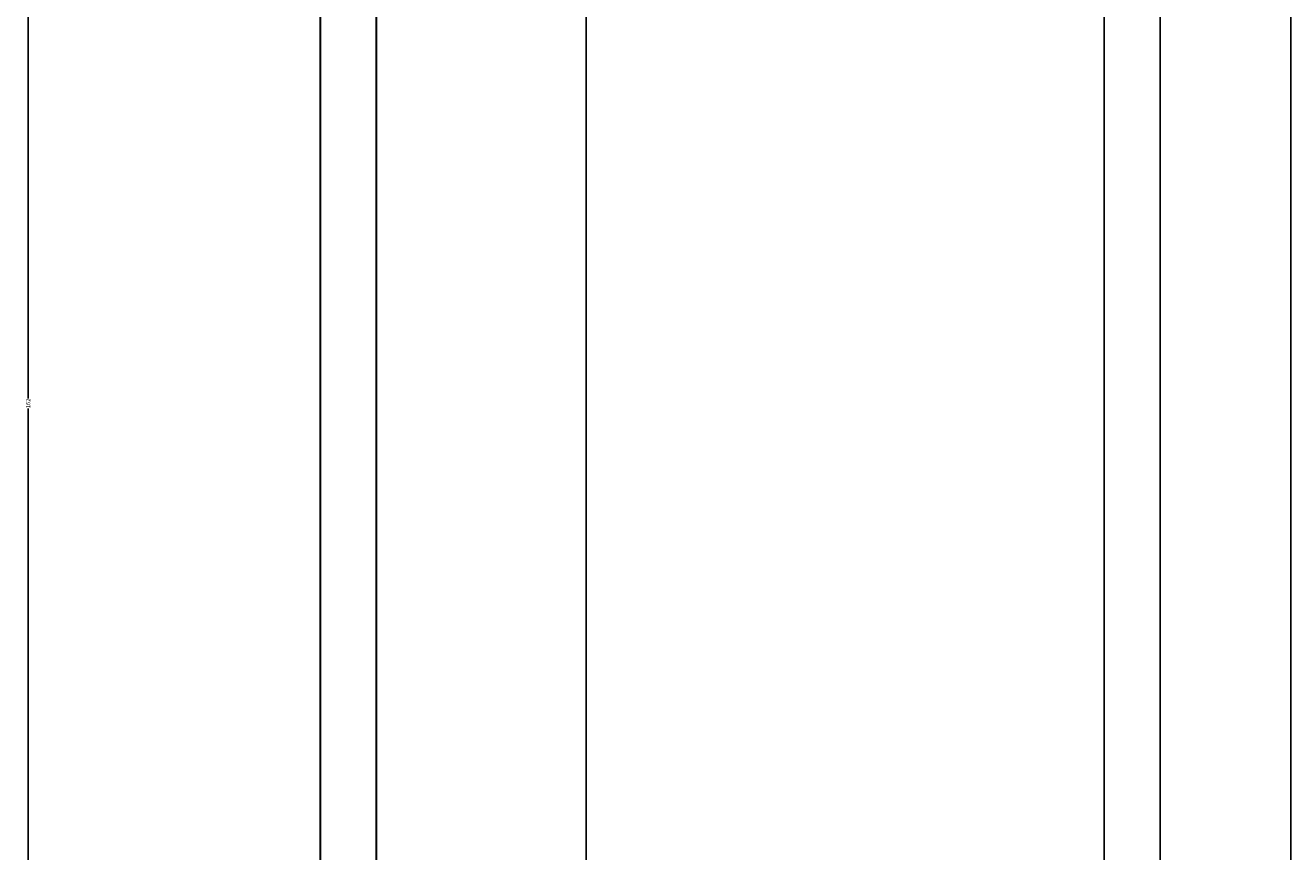
# Model space of a CAD drawing. Units: inches. Extents: x 867 to 1667, y -234 to 788.
# Tile 8 of 42: x 867 to 1071, y -8 to 125. Entities that reach past the tile are written whole.
import ezdxf

# ---------------------------------------------------------------- set-up
doc = ezdxf.new("R2010")
doc.units = ezdxf.units.IN
doc.header["$MEASUREMENT"] = 0
doc.layers.add('A-ANNO-DIMS', color=2, linetype='Continuous', lineweight=18)
doc.layers.add('A-WALL-SITE', color=8, linetype='Continuous', lineweight=30)
doc.styles.get("Standard").update_dxf_attribs({"font": 'arial.ttf'})
doc.dimstyles.get("Standard").update_dxf_attribs({"dimtxt": 0.6875, "dimasz": 0.18, "dimexe": 0.18, "dimexo": 0.0625, "dimgap": 0.09, "dimtad": 0, "dimdec": 4, "dimzin": 0, "dimdsep": 46, "dimlunit": 4, "dimtxsty": 'Standard', "dimcen": 0.09, "dimadec": 0, "dimazin": 0, "dimtfac": 1, "dimtdec": 4, "dimtofl": 0, "dimtmove": 0, "dimatfit": 3, "dimfxl": 1, "dimtolj": 1, "dimtzin": 0, "dimarcsym": 0})

# ---------------------------------------------------------------- blocks, each defined once
blk = doc.blocks.new('*D28')
at = {"layer": 'A-ANNO-DIMS', "color": 0, "lineweight": -2, "transparency": 16777216}
for p, q in [((914.89, 623.55), (914.89, -233.54)), ((957.64, 623.55), (957.64, -233.54)), ((915.07, -233.36), (935, -233.36)), ((957.46, -233.36), (937.53, -233.36))]:
    blk.add_line(p, q, dxfattribs=at)
at = {"layer": 'A-ANNO-DIMS', "color": 0, "transparency": 16777216}
for points in [[(915.07, -233.33), (915.07, -233.39), (914.89, -233.36)], [(957.46, -233.33), (957.46, -233.39), (957.64, -233.36)]]:
    blk.add_solid(points, dxfattribs=at)
at = {"layer": 'Defpoints', "color": 0, "transparency": 16777216}
for p in [(914.89, 623.62), (957.64, 623.62), (914.89, -233.36)]:
    blk.add_point(p, dxfattribs=at)
at = {"layer": 'A-ANNO-DIMS', "color": 0, "transparency": 16777216, "insert": (936.26, -233.36), "char_height": 0.688, "attachment_point": 5}
blk.add_mtext('\\A1;42.75', dxfattribs=at)
blk = doc.blocks.new('*D37')
at = {"layer": 'A-ANNO-DIMS', "color": 0, "lineweight": -2, "transparency": 16777216}
for p, q in [((1049.89, 257.55), (1049.89, -233.54)), ((1196.89, 257.55), (1196.89, -233.54)), ((1050.07, -233.36), (1122.57, -233.36)), ((1196.71, -233.36), (1124.2, -233.36))]:
    blk.add_line(p, q, dxfattribs=at)
at = {"layer": 'A-ANNO-DIMS', "color": 0, "transparency": 16777216}
for points in [[(1050.07, -233.33), (1050.07, -233.39), (1049.89, -233.36)], [(1196.71, -233.33), (1196.71, -233.39), (1196.89, -233.36)]]:
    blk.add_solid(points, dxfattribs=at)
at = {"layer": 'Defpoints', "color": 0, "transparency": 16777216}
for p in [(1049.89, 257.62), (1196.89, 257.62), (1196.89, -233.36)]:
    blk.add_point(p, dxfattribs=at)
at = {"layer": 'A-ANNO-DIMS', "color": 0, "transparency": 16777216, "insert": (1123.39, -233.36), "char_height": 0.688, "attachment_point": 5}
blk.add_mtext('\\A1;147', dxfattribs=at)
blk = doc.blocks.new('*D44')
at = {"layer": 'A-ANNO-DIMS', "color": 0, "lineweight": -2, "transparency": 16777216}
for p, q in [((1070.82, 145.12), (867.76, 145.12)), ((867.94, 144.94), (867.94, 64.93)), ((867.94, -16.7), (867.94, 63.3)), ((1070.82, -16.88), (867.76, -16.88))]:
    blk.add_line(p, q, dxfattribs=at)
at = {"layer": 'A-ANNO-DIMS', "color": 0, "transparency": 16777216}
for points in [[(867.91, 144.94), (867.97, 144.94), (867.94, 145.12)], [(867.91, -16.7), (867.97, -16.7), (867.94, -16.88)]]:
    blk.add_solid(points, dxfattribs=at)
at = {"layer": 'Defpoints', "color": 0, "transparency": 16777216}
for p in [(867.94, 145.12), (1070.89, 145.12), (1070.89, -16.88)]:
    blk.add_point(p, dxfattribs=at)
at = {"layer": 'A-ANNO-DIMS', "color": 0, "transparency": 16777216, "insert": (867.94, 64.12), "char_height": 0.688, "attachment_point": 5, "rotation": 90}
blk.add_mtext('\\A1;162', dxfattribs=at)
blk = doc.blocks.new('*D63')
at = {"layer": 'A-ANNO-DIMS', "color": 0, "lineweight": -2, "transparency": 16777216}
for p, q in [((1040.89, 257.55), (1040.89, -233.54)), ((1070.89, 221.55), (1070.89, -233.54)), ((1041.07, -233.36), (1055.31, -233.36)), ((1070.71, -233.36), (1056.47, -233.36))]:
    blk.add_line(p, q, dxfattribs=at)
at = {"layer": 'A-ANNO-DIMS', "color": 0, "transparency": 16777216}
for points in [[(1041.07, -233.33), (1041.07, -233.39), (1040.89, -233.36)], [(1070.71, -233.33), (1070.71, -233.39), (1070.89, -233.36)]]:
    blk.add_solid(points, dxfattribs=at)
at = {"layer": 'Defpoints', "color": 0, "transparency": 16777216}
for p in [(1040.89, 257.62), (1070.89, 221.62), (1070.89, -233.36)]:
    blk.add_point(p, dxfattribs=at)
at = {"layer": 'A-ANNO-DIMS', "color": 0, "transparency": 16777216, "insert": (1055.89, -233.36), "char_height": 0.688, "attachment_point": 5}
blk.add_mtext('\\A1;30', dxfattribs=at)

msp = doc.modelspace()

# ---------------------------------------------------------------- linework, layer by layer
at = {"layer": 'A-WALL-SITE'}
for p, q in [((914.8866, 740.617), (914.8866, -186.4081)), ((923.8866, 740.617), (923.8866, -186.4081))]:
    msp.add_line(p, q, dxfattribs=at)

# ---------------------------------------------------------------- dimensions: what is measured, and where the dimension line sits
at = {"layer": 'A-ANNO-DIMS'}
for base, p1, p2, override, picture, middle in [((914.8866, -233.3581), (957.6375, 623.617), (914.8866, 623.617), {"dimdec": 2, "dimlfac": 1, "dimrnd": 0, "dimzin": 0, "dimdsep": 46, "dimlunit": 2}, '*D28', (936.2621, -233.3581)), ((1070.8866, -233.3581), (1040.8866, 257.617), (1070.8866, 221.617), {"dimdec": 0, "dimlfac": 1, "dimrnd": 0, "dimzin": 0, "dimdsep": 46, "dimlunit": 2}, '*D63', (1055.8866, -233.3581)), ((1196.8866, -233.3581), (1049.8866, 257.617), (1196.8866, 257.617), {"dimdec": 0, "dimlfac": 1, "dimrnd": 0, "dimzin": 0, "dimdsep": 46, "dimlunit": 2}, '*D37', (1123.3866, -233.3581))]:
    dim = msp.add_linear_dim(base=base, p1=p1, p2=p2, dimstyle='Standard', override=override, dxfattribs=at)
    dim.commit()
    dim.dimension.update_dxf_attribs({"geometry": picture, "text_midpoint": middle})
dim = msp.add_linear_dim(base=(867.9366, 145.117), p1=(1070.8866, -16.883), p2=(1070.8866, 145.117), angle=90, dimstyle='Standard', override={"dimdec": 0, "dimlfac": 1, "dimrnd": 0, "dimzin": 0, "dimdsep": 46, "dimlunit": 2}, dxfattribs=at)
dim.commit()
dim.dimension.update_dxf_attribs({"geometry": '*D44', "text_midpoint": (867.9366, 64.117)})

doc.saveas('drawing.dxf')
